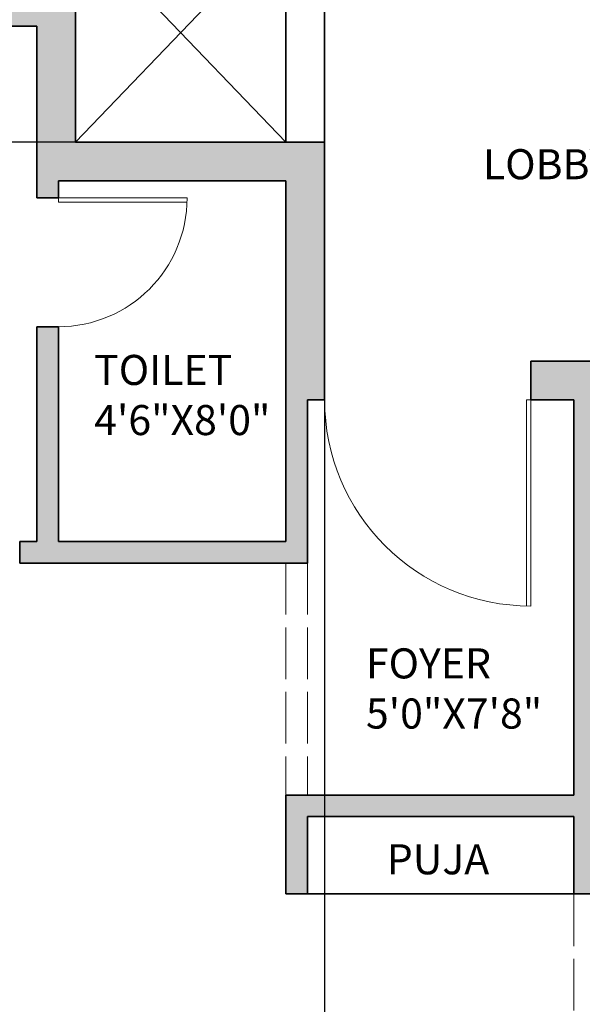
# Model space of a CAD drawing. Units: inches. Extents: x 2540 to 3167, y 3083 to 4007.
# Tile 6 of 15: x 2798 to 2929, y 3313 to 3542. Entities that reach past the tile are written whole.
import ezdxf

# ---------------------------------------------------------------- set-up
doc = ezdxf.new("R2010")
doc.units = ezdxf.units.IN
doc.linetypes.add('ACAD_ISO02W100', pattern=[15, 12, -3])
for name, color, linetype, lineweight in [('A-ANNO-DIMS', 2, 'Continuous', 18), ('A-AREA-IDEN', 7, 'Continuous', 18), ('A-DOOR', 4, 'Continuous', 18), ('A-FLOR-OPEN', 8, 'Continuous', 13)]:
    doc.layers.add(name, color=color, linetype=linetype, lineweight=lineweight)
for name, color, linetype, lineweight, true_color in [('A-WALL', 143, 'Continuous', 35, 0x7aafdf), ('A-WALL-OVHD', 143, 'ACAD_ISO02W100', 18, 0x7aafdf), ('A-WALL-PATT', 143, 'Continuous', 13, 0x7aafdf)]:
    doc.layers.add(name, color=color, linetype=linetype, lineweight=lineweight, true_color=true_color)
doc.styles.get("Standard").update_dxf_attribs({"font": 'arial.ttf'})
doc.dimstyles.get("Standard").update_dxf_attribs({"dimtxt": 0.18, "dimasz": 0.18, "dimexe": 0.18, "dimexo": 0.0625, "dimgap": 0.09, "dimtad": 0, "dimtih": 1, "dimtoh": 1, "dimdec": 4, "dimzin": 0, "dimdsep": 46, "dimtxsty": 'Standard', "dimcen": 0.09, "dimadec": 0, "dimazin": 0, "dimtfac": 1, "dimtdec": 4, "dimtofl": 0, "dimtmove": 0, "dimatfit": 3, "dimfxl": 1, "dimtolj": 1, "dimtzin": 0, "dimarcsym": 0})

# ---------------------------------------------------------------- blocks, each defined once
blk = doc.blocks.new('*D44')
at = {"layer": 'A-ANNO-DIMS', "color": 0, "lineweight": -2, "transparency": 16777216}
for p, q in [((2771.45, 3964.71), (2540.23, 3964.71)), ((2540.41, 3964.53), (2540.41, 3545.4)), ((2540.41, 3125.89), (2540.41, 3545.03)), ((2810.45, 3125.71), (2540.23, 3125.71))]:
    blk.add_line(p, q, dxfattribs=at)
at = {"layer": 'A-ANNO-DIMS', "color": 0, "transparency": 16777216}
for points in [[(2540.38, 3964.53), (2540.44, 3964.53), (2540.41, 3964.71)], [(2540.38, 3125.89), (2540.44, 3125.89), (2540.41, 3125.71)]]:
    blk.add_solid(points, dxfattribs=at)
at = {"layer": 'Defpoints', "color": 0, "transparency": 16777216}
for p in [(2540.41, 3964.71), (2771.51, 3964.71), (2810.51, 3125.71)]:
    blk.add_point(p, dxfattribs=at)
at = {"layer": 'A-ANNO-DIMS', "color": 0, "transparency": 16777216, "insert": (2540.41, 3545.21), "char_height": 0.18, "attachment_point": 5}
blk.add_mtext('\\A1;839', dxfattribs=at)
blk = doc.blocks.new('*D55')
at = {"layer": 'A-ANNO-DIMS', "color": 0, "lineweight": -2, "transparency": 16777216}
for p, q in [((2868.51, 3564.65), (2868.51, 3083.43)), ((2930.51, 3543.65), (2930.51, 3083.43)), ((2868.69, 3083.61), (2899.29, 3083.61)), ((2930.33, 3083.61), (2899.73, 3083.61))]:
    blk.add_line(p, q, dxfattribs=at)
at = {"layer": 'A-ANNO-DIMS', "color": 0, "transparency": 16777216}
for points in [[(2868.69, 3083.64), (2868.69, 3083.58), (2868.51, 3083.61)], [(2930.33, 3083.64), (2930.33, 3083.58), (2930.51, 3083.61)]]:
    blk.add_solid(points, dxfattribs=at)
at = {"layer": 'Defpoints', "color": 0, "transparency": 16777216}
for p in [(2868.51, 3564.71), (2930.51, 3543.71), (2930.51, 3083.61)]:
    blk.add_point(p, dxfattribs=at)
at = {"layer": 'A-ANNO-DIMS', "color": 0, "transparency": 16777216, "insert": (2899.51, 3083.61), "char_height": 0.18, "attachment_point": 5}
blk.add_mtext('\\A1;62', dxfattribs=at)
blk = doc.blocks.new('*D57')
at = {"layer": 'A-ANNO-DIMS', "color": 0, "lineweight": -2, "transparency": 16777216}
for p, q in [((2810.45, 3564.71), (2540.23, 3564.71)), ((2540.41, 3564.53), (2540.41, 3539.4)), ((2540.41, 3513.89), (2540.41, 3539.03)), ((2810.45, 3513.71), (2540.23, 3513.71))]:
    blk.add_line(p, q, dxfattribs=at)
at = {"layer": 'A-ANNO-DIMS', "color": 0, "transparency": 16777216}
for points in [[(2540.38, 3564.53), (2540.44, 3564.53), (2540.41, 3564.71)], [(2540.38, 3513.89), (2540.44, 3513.89), (2540.41, 3513.71)]]:
    blk.add_solid(points, dxfattribs=at)
at = {"layer": 'Defpoints', "color": 0, "transparency": 16777216}
for p in [(2810.51, 3564.71), (2540.41, 3513.71), (2810.51, 3513.71)]:
    blk.add_point(p, dxfattribs=at)
at = {"layer": 'A-ANNO-DIMS', "color": 0, "transparency": 16777216, "insert": (2540.41, 3539.21), "char_height": 0.18, "attachment_point": 5}
blk.add_mtext('\\A1;51', dxfattribs=at)

msp = doc.modelspace()

# ---------------------------------------------------------------- hatches: boundary and pattern name
at = {"layer": 'A-WALL-PATT'}
h = msp.add_hatch(color=256, dxfattribs=at)
h.dxf.hatch_style = 1
h.paths.add_polyline_path([(2805.51, 3803.71), (2800.51, 3803.71), (2800.51, 3799.71), (2621.51, 3799.71), (2621.51, 3823.71), (2612.51, 3823.71), (2612.51, 3794.71), (2636.51, 3794.71), (2636.51, 3782.71), (2645.51, 3782.71), (2645.51, 3794.71), (2805.51, 3794.71)])
h.paths.add_polyline_path([(2810.51, 3564.71), (2868.51, 3564.71), (2868.51, 3627.71), (2872.51, 3627.71), (2872.51, 3636.71), (2864.51, 3636.71), (2864.51, 3674.71), (2797.51, 3674.71), (2797.51, 3669.71), (2801.51, 3669.71), (2801.51, 3628.63), (2806.51, 3628.63), (2806.51, 3669.71), (2859.51, 3669.71), (2859.51, 3573.71), (2806.51, 3573.71), (2806.51, 3598.63), (2801.51, 3598.63), (2801.51, 3549.71), (2645.51, 3549.71), (2645.51, 3573.71), (2636.51, 3573.71), (2636.51, 3516.71), (2645.51, 3516.71), (2645.51, 3540.71), (2801.51, 3540.71), (2801.51, 3504.71), (2801.51, 3500.71), (2806.51, 3500.71), (2806.51, 3504.71), (2859.51, 3504.71), (2859.51, 3420.71), (2806.51, 3420.71), (2806.51, 3470.71), (2801.51, 3470.71), (2801.51, 3420.71), (2797.51, 3420.71), (2797.51, 3415.71), (2864.51, 3415.71), (2864.51, 3453.71), (2868.51, 3453.71), (2868.51, 3513.71), (2810.51, 3513.71)])
h.paths.add_polyline_path([(2645.51, 3415.71), (2761.51, 3415.71), (2761.51, 3420.71), (2645.51, 3420.71), (2645.51, 3444.71), (2636.51, 3444.71), (2636.51, 3403.71), (2645.51, 3403.71)])
h.paths.add_polyline_path([(2645.51, 3307.71), (2636.51, 3307.71), (2636.51, 3295.71), (2612.51, 3295.71), (2612.51, 3149.71), (2645.51, 3149.71), (2645.51, 3158.71), (2621.51, 3158.71), (2621.51, 3290.71), (2801.51, 3290.71), (2801.51, 3286.71), (2806.51, 3286.71), (2806.51, 3295.71), (2645.51, 3295.71)])
h.paths.add_polyline_path([(2762.01, 3158.71), (2746.51, 3158.71), (2746.51, 3240.71), (2750.51, 3240.71), (2750.51, 3245.71), (2741.51, 3245.71), (2741.51, 3158.71), (2717.51, 3158.71), (2717.51, 3149.71), (2762.01, 3149.71)], flags=17)
h.paths.add_polyline_path([(2810.51, 3173.71), (2822.51, 3173.71), (2822.51, 3182.71), (2806.51, 3182.71), (2806.51, 3250.71), (2801.51, 3250.71), (2801.51, 3245.71), (2780.51, 3245.71), (2780.51, 3240.71), (2801.51, 3240.71), (2801.51, 3158.71), (2786.01, 3158.71), (2786.01, 3149.71), (2810.51, 3149.71)])
h.paths.add_polyline_path([(2931.51, 3290.71), (2935.51, 3290.71), (2935.51, 3295.71), (2926.51, 3295.71), (2926.51, 3182.71), (2910.51, 3182.71), (2910.51, 3173.71), (2922.51, 3173.71), (2922.51, 3149.71), (2987.51, 3149.71), (2987.51, 3158.71), (2931.51, 3158.71)])
h.paths.add_polyline_path([(3124.51, 3295.71), (3086.51, 3295.71), (3018.51, 3295.71), (3018.51, 3290.71), (3115.51, 3290.71), (3115.51, 3158.71), (3059.51, 3158.71), (3059.51, 3149.71), (3124.51, 3149.71)])
h.paths.add_polyline_path([(2988.51, 3295.71), (2984.51, 3295.71), (2984.51, 3349.71), (3086.51, 3349.71), (3086.51, 3320.71), (3124.51, 3320.71), (3124.51, 3354.71), (3071.51, 3354.71), (3071.51, 3358.71), (3062.51, 3358.71), (3062.51, 3354.71), (2979.51, 3354.71), (2979.51, 3295.71), (2971.51, 3295.71), (2971.51, 3290.71), (2988.51, 3290.71)])
h.paths.add_polyline_path([(3095.51, 3325.71), (3095.51, 3349.71), (3119.51, 3349.71), (3119.51, 3325.71)], flags=16)
h.paths.add_polyline_path([(3124.51, 3462.71), (3071.51, 3462.71), (3071.51, 3627.71), (3124.51, 3627.71), (3124.51, 3693.71), (3095.51, 3693.71), (3095.51, 3702.71), (3086.51, 3702.71), (3086.51, 3684.71), (3086.51, 3636.71), (2930.51, 3636.71), (2930.51, 3768.71), (2934.51, 3768.71), (2934.51, 3773.71), (2930.51, 3773.71), (2925.51, 3773.71), (2925.51, 3730.71), (2864.51, 3730.71), (2864.51, 3760.71), (2859.51, 3760.71), (2859.51, 3725.71), (2925.51, 3725.71), (2925.51, 3636.71), (2908.51, 3636.71), (2908.51, 3627.71), (3062.51, 3627.71), (3062.51, 3543.71), (2930.51, 3543.71), (2930.51, 3534.71), (2993.51, 3534.71), (2993.51, 3516.71), (3002.51, 3516.71), (3002.51, 3534.71), (3062.51, 3534.71), (3062.51, 3462.71), (3002.51, 3462.71), (3002.51, 3480.71), (2993.51, 3480.71), (2993.51, 3462.71), (2916.51, 3462.71), (2916.51, 3453.71), (2926.51, 3453.71), (2926.51, 3361.71), (2859.51, 3361.71), (2859.51, 3338.71), (2864.51, 3338.71), (2864.51, 3356.71), (2926.51, 3356.71), (2926.51, 3338.71), (2931.51, 3338.71), (2931.51, 3453.71), (3062.51, 3453.71), (3062.51, 3448.21), (3071.51, 3448.21), (3071.51, 3453.71), (3124.51, 3453.71)])

# ---------------------------------------------------------------- linework, layer by layer
at = {"layer": 'A-DOOR'}
for p, q in [((2806.51, 3500.71), (2836.51, 3500.71)), ((2806.51, 3500.71), (2806.51, 3499.71)), ((2806.51, 3499.71), (2836.49, 3499.71)), ((2915.51, 3453.71), (2915.51, 3405.72)), ((2916.51, 3453.71), (2915.51, 3453.71)), ((2916.51, 3453.71), (2916.51, 3405.71))]:
    msp.add_line(p, q, dxfattribs=at)
for centre, radius, start, end in [((2806.45, 3500.77), 30.06, 270.1094, 359.8906), ((2916.51, 3453.71), 48, 180, 270)]:
    msp.add_arc(centre, radius, start, end, dxfattribs=at)
at = {"layer": 'A-FLOR-OPEN'}
for p, q in [((2859.51, 3513.71), (2810.51, 3564.71)), ((2810.51, 3513.71), (2859.51, 3564.71))]:
    msp.add_line(p, q, dxfattribs=at)
at = {"layer": 'A-WALL'}
for p, q in [((2868.51, 3627.71), (2868.51, 3453.71)), ((2810.51, 3564.71), (2810.51, 3513.71)), ((2859.51, 3564.71), (2859.51, 3513.71)), ((2645.51, 3540.71), (2801.51, 3540.71)), ((2801.51, 3540.71), (2801.51, 3504.71)), ((2810.51, 3513.71), (2868.51, 3513.71)), ((2801.51, 3504.71), (2801.51, 3500.71)), ((2806.51, 3504.71), (2859.51, 3504.71)), ((2806.51, 3504.71), (2806.51, 3500.71)), ((2859.51, 3504.71), (2859.51, 3420.71)), ((2801.51, 3500.71), (2806.51, 3500.71)), ((2801.51, 3470.71), (2806.51, 3470.71)), ((2801.51, 3470.71), (2801.51, 3420.71)), ((2806.51, 3470.71), (2806.51, 3420.71)), ((2916.51, 3462.71), (2993.51, 3462.71)), ((2916.51, 3462.71), (2916.51, 3453.71)), ((2864.51, 3453.71), (2868.51, 3453.71)), ((2864.51, 3453.71), (2864.51, 3415.71)), ((2916.51, 3453.71), (2926.51, 3453.71)), ((2926.51, 3453.71), (2926.51, 3361.71)), ((2797.51, 3420.71), (2797.51, 3415.71)), ((2797.51, 3420.71), (2801.51, 3420.71)), ((2806.51, 3420.71), (2859.51, 3420.71)), ((2797.51, 3415.71), (2864.51, 3415.71)), ((2859.51, 3361.71), (2926.51, 3361.71)), ((2859.51, 3361.71), (2859.51, 3338.71)), ((2864.51, 3356.71), (2926.51, 3356.71)), ((2864.51, 3356.71), (2864.51, 3338.71)), ((2926.51, 3356.71), (2926.51, 3338.56)), ((2859.51, 3338.71), (2931.51, 3338.71))]:
    msp.add_line(p, q, dxfattribs=at)
at = {"layer": 'A-WALL-OVHD'}
for p, q in [((2859.51, 3415.71), (2859.51, 3361.71)), ((2864.51, 3415.71), (2864.51, 3361.71)), ((2926.51, 3338.56), (2926.51, 3295.71))]:
    msp.add_line(p, q, dxfattribs=at)

# ---------------------------------------------------------------- texts
at = {"layer": 'A-AREA-IDEN', "char_height": 7, "attachment_point": 1}
for s, width, insert in [('LOBBY', 34.4573, (2905.37, 3512.07)), ('TOILET\\P4\'6"X8\'0"', 75.6369, (2814.86, 3464.18)), ('FOYER\\P5\'0"X7\'8"', 38.2617, (2878.14, 3395.86)), ('PUJA', 34.4573, (2882.99, 3350.26))]:
    msp.add_mtext_dynamic_manual_height_columns(s, width=width, gutter_width=12.5, heights=[0], dxfattribs=dict(at, insert=insert))

# ---------------------------------------------------------------- dimensions: what is measured, and where the dimension line sits
at = {"layer": 'A-ANNO-DIMS'}
for base, p1, p2, picture, middle in [((2540.41, 3964.71), (2810.51, 3125.71), (2771.51, 3964.71), '*D44', (2540.41, 3545.21)), ((2540.41, 3513.71), (2810.51, 3564.71), (2810.51, 3513.71), '*D57', (2540.41, 3539.21))]:
    dim = msp.add_linear_dim(base=base, p1=p1, p2=p2, angle=90, dimstyle='Standard', override={"dimdec": 0, "dimlfac": 1, "dimrnd": 0, "dimzin": 0, "dimdsep": 46, "dimlunit": 2}, dxfattribs=at)
    dim.commit()
    dim.dimension.update_dxf_attribs({"geometry": picture, "text_midpoint": middle})
dim = msp.add_linear_dim(base=(2930.51, 3083.61), p1=(2868.51, 3564.71), p2=(2930.51, 3543.71), dimstyle='Standard', override={"dimdec": 0, "dimlfac": 1, "dimrnd": 0, "dimzin": 0, "dimdsep": 46, "dimlunit": 2}, dxfattribs=at)
dim.commit()
dim.dimension.update_dxf_attribs({"geometry": '*D55', "text_midpoint": (2899.51, 3083.61)})

doc.saveas('drawing.dxf')
